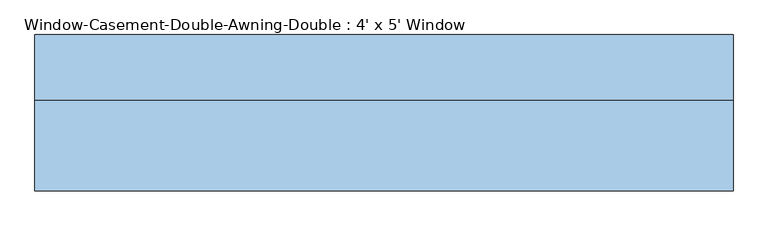
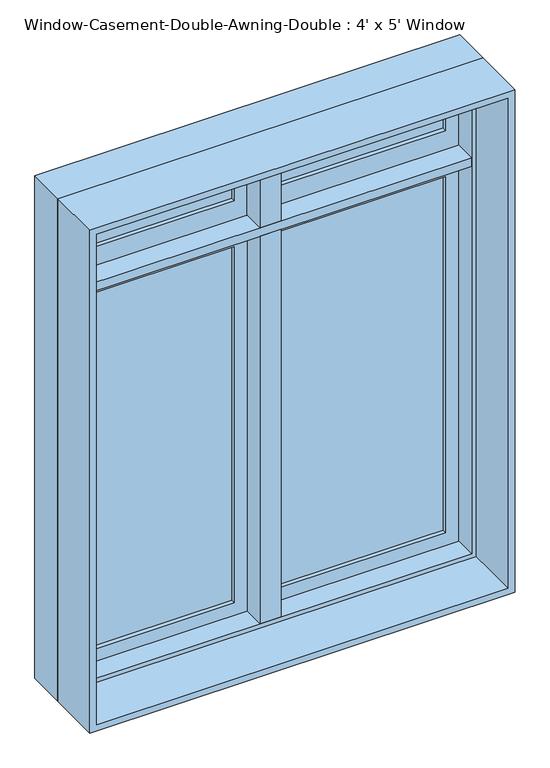
"""IFC4 building model written with IfcOpenShell, lengths in millimetres: window geometry, Window-Casement-Double-Awning-Double : 4' x 5' Window."""

from ifc_helpers import new_model, si_unit, frame, origin, place, context, project, spatial, polyline, outline, extrude, faceted_brep, source, transform, mapped, element, save


def window_casement_double_awning_double_4_x_5_window_c6f36ef5(model_context):
    return source(origin(), model_context, "Body", "SolidModel", [
        faceted_brep([(577.85, 95.25, 2406.65), (577.85, 31.75, 2406.65), (-577.85, 31.75, 2406.65), (-577.85, 95.25, 2406.65), (596.9, 146.05, 2425.7), (596.9, 95.25, 2425.7), (-596.9, 95.25, 2425.7), (-596.9, 146.05, 2425.7), (609.6, 31.75, 2438.4), (609.6, 146.05, 2438.4), (-609.6, 146.05, 2438.4), (-609.6, 31.75, 2438.4), (-577.85, 31.75, 946.15), (-577.85, 95.25, 946.15), (-596.9, 95.25, 927.1), (-596.9, 146.05, 927.1), (-609.6, 146.05, 914.4), (-609.6, 31.75, 914.4), (577.85, 31.75, 946.15), (577.85, 95.25, 946.15), (596.9, 95.25, 927.1), (596.9, 146.05, 927.1), (609.6, 146.05, 914.4), (609.6, 31.75, 914.4)], [[[0, 1, 2, 3]], [[4, 5, 6, 7]], [[8, 9, 10, 11]], [[3, 2, 12, 13]], [[7, 6, 14, 15]], [[11, 10, 16, 17]], [[13, 12, 18, 19]], [[15, 14, 20, 21]], [[17, 16, 22, 23]], [[11, 17, 23, 8], [1, 18, 12, 2]], [[19, 18, 1, 0]], [[5, 20, 14, 6], [3, 13, 19, 0]], [[21, 20, 5, 4]], [[23, 22, 9, 8]], [[9, 22, 16, 10], [7, 15, 21, 4]]]),
        extrude(outline(polyline([(2438.4, -609.6), (914.4, -609.6), (914.4, 609.6), (2438.4, 609.6), (2438.4, -609.6)]), holes=[polyline([(2419.35, 590.55), (933.45, 590.55), (933.45, -590.55), (2419.35, -590.55), (2419.35, 590.55)])]), frame((0.0, -127.0, 0.0), z_axis=(0.0, 1.0, 0.0), x_axis=(0.0, 0.0, 1.0)), (0.0, 0.0, 1.0), 158.75),
        extrude(outline(polyline([(927.1, 596.9), (2120.9, 596.9), (2120.9, 9.525), (927.1, 9.525), (927.1, 596.9)]), holes=[polyline([(984.25, 66.675), (2063.75, 66.675), (2063.75, 539.75), (984.25, 539.75), (984.25, 66.675)])]), frame((0.0, 95.25, 0.0), z_axis=(0.0, 1.0, 0.0), x_axis=(0.0, 0.0, 1.0)), (0.0, 0.0, 1.0), 44.45),
        extrude(outline(polyline([(2120.9, -596.9), (927.1, -596.9), (927.1, -9.525), (2120.9, -9.525), (2120.9, -596.9)]), holes=[polyline([(2063.75, -66.675), (984.25, -66.675), (984.25, -539.75), (2063.75, -539.75), (2063.75, -66.675)])]), frame((0.0, 95.25, 0.0), z_axis=(0.0, 1.0, 0.0), x_axis=(0.0, 0.0, 1.0)), (0.0, 0.0, 1.0), 44.45),
        extrude(outline(polyline([(539.75, 127.0), (539.75, 120.65), (66.675, 120.65), (66.675, 127.0), (539.75, 127.0)])), frame((0.0, 0.0, 984.25), z_axis=(0.0, 0.0, 1.0), x_axis=(1.0, 0.0, 0.0)), (0.0, 0.0, 1.0), 1079.5),
        extrude(outline(polyline([(66.675, 107.95), (66.675, 114.3), (539.75, 114.3), (539.75, 107.95), (66.675, 107.95)])), frame((0.0, 0.0, 984.25), z_axis=(0.0, 0.0, 1.0), x_axis=(1.0, 0.0, 0.0)), (0.0, 0.0, 1.0), 1079.5),
        extrude(outline(polyline([(-66.675, 127.0), (-66.675, 120.65), (-539.75, 120.65), (-539.75, 127.0), (-66.675, 127.0)])), frame((0.0, 0.0, 984.25), z_axis=(0.0, 0.0, 1.0), x_axis=(1.0, 0.0, 0.0)), (0.0, 0.0, 1.0), 1079.5),
        extrude(outline(polyline([(-539.75, 107.95), (-539.75, 114.3), (-66.675, 114.3), (-66.675, 107.95), (-539.75, 107.95)])), frame((0.0, 0.0, 984.25), z_axis=(0.0, 0.0, 1.0), x_axis=(1.0, 0.0, 0.0)), (0.0, 0.0, 1.0), 1079.5),
        faceted_brep([(9.525, 146.05, 2120.9), (-9.525, 146.05, 2120.9), (-9.525, 95.25, 2120.9), (-30.1625, 95.25, 2120.9), (-30.1625, 31.75, 2120.9), (30.1625, 31.75, 2120.9), (30.1625, 95.25, 2120.9), (9.525, 95.25, 2120.9), (9.525, 146.05, 927.1), (9.525, 95.25, 927.1), (-9.525, 95.25, 927.1), (-9.525, 146.05, 927.1), (-9.525, 95.25, 946.15), (-30.1625, 95.25, 946.15), (-30.1625, 31.75, 946.15), (30.1625, 31.75, 946.15), (30.1625, 95.25, 946.15), (9.525, 95.25, 946.15)], [[[0, 1, 2, 3, 4, 5, 6, 7]], [[8, 9, 10, 11]], [[1, 0, 8, 11]], [[2, 1, 11, 10, 12]], [[3, 2, 12, 13]], [[4, 3, 13, 14]], [[5, 4, 14, 15]], [[6, 5, 15, 16]], [[7, 6, 16, 17]], [[0, 7, 17, 9, 8]], [[17, 12, 10, 9]], [[12, 17, 16, 15, 14, 13]]]),
        extrude(outline(polyline([(-66.675, 127.0), (-66.675, 120.65), (-539.75, 120.65), (-539.75, 127.0), (-66.675, 127.0)])), frame((0.0, 0.0, 2203.45), z_axis=(0.0, 0.0, 1.0), x_axis=(1.0, 0.0, 0.0)), (0.0, 0.0, 1.0), 165.1),
        extrude(outline(polyline([(-539.75, 107.95), (-539.75, 114.3), (-66.675, 114.3), (-66.675, 107.95), (-539.75, 107.95)])), frame((0.0, 0.0, 2203.45), z_axis=(0.0, 0.0, 1.0), x_axis=(1.0, 0.0, 0.0)), (0.0, 0.0, 1.0), 165.1),
        extrude(outline(polyline([(596.9, 146.05), (596.9, 95.25), (577.85, 95.25), (577.85, 31.75), (-577.85, 31.75), (-577.85, 95.25), (-596.9, 95.25), (-596.9, 146.05), (596.9, 146.05)])), frame((0.0, 0.0, 2120.9), z_axis=(0.0, 0.0, 1.0), x_axis=(1.0, 0.0, 0.0)), (0.0, 0.0, 1.0), 25.4),
        faceted_brep([(9.525, 95.25, 2425.7), (9.525, 146.05, 2425.7), (-9.525, 146.05, 2425.7), (-9.525, 95.25, 2425.7), (-9.525, 95.25, 2146.3), (-9.525, 146.05, 2146.3), (9.525, 146.05, 2146.3), (9.525, 95.25, 2146.3), (30.1625, 95.25, 2146.3), (30.1625, 31.75, 2146.3), (-30.1625, 31.75, 2146.3), (-30.1625, 95.25, 2146.3), (-30.1625, 95.25, 2406.65), (-9.525, 95.25, 2406.65), (-30.1625, 31.75, 2406.65), (30.1625, 31.75, 2406.65), (30.1625, 95.25, 2406.65), (9.525, 95.25, 2406.65)], [[[0, 1, 2, 3]], [[4, 5, 6, 7, 8, 9, 10, 11]], [[4, 11, 12, 13]], [[11, 10, 14, 12]], [[10, 9, 15, 14]], [[9, 8, 16, 15]], [[8, 7, 17, 16]], [[1, 0, 17, 7, 6]], [[2, 1, 6, 5]], [[3, 2, 5, 4, 13]], [[17, 13, 12, 14, 15, 16]], [[13, 17, 0, 3]]]),
        extrude(outline(polyline([(2425.7, 9.525), (2146.3, 9.525), (2146.3, 596.9), (2425.7, 596.9), (2425.7, 9.525)]), holes=[polyline([(2368.55, 539.75), (2203.45, 539.75), (2203.45, 66.675), (2368.55, 66.675), (2368.55, 539.75)])]), frame((0.0, 95.25, 0.0), z_axis=(0.0, 1.0, 0.0), x_axis=(0.0, 0.0, 1.0)), (0.0, 0.0, 1.0), 44.45),
        extrude(outline(polyline([(2146.3, -9.525), (2425.7, -9.525), (2425.7, -596.9), (2146.3, -596.9), (2146.3, -9.525)]), holes=[polyline([(2203.45, -539.75), (2368.55, -539.75), (2368.55, -66.675), (2203.45, -66.675), (2203.45, -539.75)])]), frame((0.0, 95.25, 0.0), z_axis=(0.0, 1.0, 0.0), x_axis=(0.0, 0.0, 1.0)), (0.0, 0.0, 1.0), 44.45),
        extrude(outline(polyline([(66.675, 127.0), (539.75, 127.0), (539.75, 120.65), (66.675, 120.65), (66.675, 127.0)])), frame((0.0, 0.0, 2203.45), z_axis=(0.0, 0.0, 1.0), x_axis=(1.0, 0.0, 0.0)), (0.0, 0.0, 1.0), 165.1),
        extrude(outline(polyline([(539.75, 107.95), (66.675, 107.95), (66.675, 114.3), (539.75, 114.3), (539.75, 107.95)])), frame((0.0, 0.0, 2203.45), z_axis=(0.0, 0.0, 1.0), x_axis=(1.0, 0.0, 0.0)), (0.0, 0.0, 1.0), 165.1),
    ])


if __name__ == "__main__":
    model = new_model("IFC4")
    model_context = context("Model", 3, world=origin())
    ifc_project = project(units=[si_unit("LENGTHUNIT", "METRE", prefix="MILLI")], contexts=[model_context])
    site = spatial("IfcSite", under=ifc_project)
    building = spatial("IfcBuilding", under=site)
    placement = place(None, origin())
    window_casement_double_awning_double_4_x_5_window_shape = window_casement_double_awning_double_4_x_5_window_c6f36ef5(model_context)
    element("IfcWindow", 1, ObjectType="Window-Casement-Double-Awning-Double : 4' x 5' Window", at=placement, inside=building, context=model_context, shape_type="MappedRepresentation", body=[
        mapped(window_casement_double_awning_double_4_x_5_window_shape, transform((0.0, 0.0, 0.0), x_axis=(1.0, 0.0, 0.0), y_axis=(0.0, 1.0, 0.0), z_axis=(0.0, 0.0, 1.0))),
    ])
    save(model, "model.ifc")

# Revit data of these elements
# Type "Window-Casement-Double-Awning-Double : 4' x 5' Window"
#   Type Mark = "19"
#   Fire Rating = "0.5h"
#   Assembly Code = "B2020100"
#   Analytic Construction = "Double glazing - domestic"
#   Window Inset [instance default] = 0' - 0"
#   Wall Thickness [instance default] = 0' - 6"
#   Interior Wall Closure [instance default] = 0' - 2 1/4"
#   Half Width = 2' - 0"
#   Visual Light Transmittance = 0.81
#   Transom Height = 1' - 0"
#   Thermal Resistance (R) = 1.8146 (h·ft²·°F)/BTU
#   Solar Heat Gain Coefficient = 0.76
#   Rough Width = 4' - 0 1/2"
#   Rough Height = 5' - 0 1/2"
#   Open Window Height = 4' - 0"
#   Frame Extension [instance default] = 0' - 0 1/4"
#   Height = 5' - 0"
#   Heat Transfer Coefficient (U) = 0.5511 BTU/(h·ft²·°F)
#   Exterior Wall Closure [instance default] = 0' - 1 1/4"
#   Extension Jamb [instance default] = 0' - 2 1/4"
#   Default Sill Height = 3' - 0"
#   Width = 4' - 0"
#   Top Muntin Visibility = yes
#   Bottom Muntin Visibility = yes
#   Interior Trim Visibility [instance default] = yes
#   Exterior Trim Visibility [instance default] = yes
#   Extension Jamb Visibility [instance default] = yes
#   Interior Trim Material = Wood - Stained
#   Muntin Pattern = Muntin Pattern_2x2 : Muntin Pattern_2x2
#   Interior Trim = Trim-Window-Interior-Flat : Picture Frame
#   Interior Frame Material = Wood - Stained
#   Glass Panel Material = Glass
#   Exterior Trim Material = Clad - White
#   Exterior Trim = Trim-Window-Exterior-Flat : with Sill
#   Exterior Frame Material = Clad - White
#   Wall Closure = (empty or 0)
# Element 1 (IfcWindow, "Window-Casement-Double-Awning-Double : 4' x 5' Window")
#   Wall Thickness = 0' - 10"
#   Extension Jamb = 0' - 6 1/4"
#   Materials on its faces: "Wood - Stained", "Glass", "Clad - White"
# Materials
#   "Wood - Stained": class "Wood", colour RGB 224 178 126, transparency 0, Cost = 0
#   "Glass": class "Glass", colour RGB 0 128 192, transparency 0.75, Description = "Soda Lime Glass", Cost = 0
#   "Clad - White": class "Wood", colour RGB 242 242 238, transparency 0, Cost = 0
